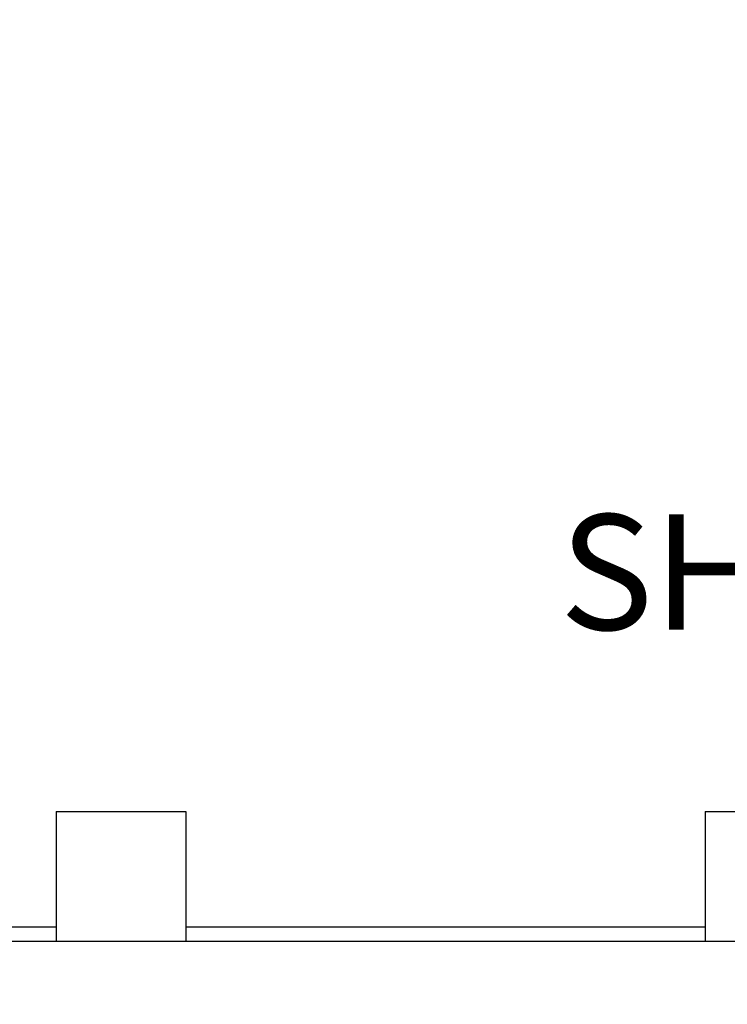
# Model space of a CAD drawing. Units: inches. Extents: x -48 to 50072, y 0 to 21068.
# Tile 4 of 75: x 163 to 212, y 210 to 278. Entities that reach past the tile are written whole.
import ezdxf

# ---------------------------------------------------------------- set-up
doc = ezdxf.new("R2010")
doc.units = ezdxf.units.IN
doc.header["$MEASUREMENT"] = 0
doc.layers.add('A-ANNO-DIMS', color=2, linetype='Continuous', lineweight=18)
doc.layers.add('C-PROP', color=7, linetype='Continuous', lineweight=25)
doc.styles.get("Standard").update_dxf_attribs({"font": 'arial.ttf'})
doc.dimstyles.get("Standard").update_dxf_attribs({"dimtxt": 8, "dimasz": 0.18, "dimexe": 0.18, "dimexo": 0.0625, "dimgap": 0.09, "dimtad": 0, "dimtih": 1, "dimtoh": 1, "dimdec": 1, "dimzin": 0, "dimdsep": 46, "dimlunit": 4, "dimtxsty": 'Standard', "dimblk": 'ARCHTICK', "dimcen": 0.09, "dimadec": 0, "dimazin": 0, "dimtfac": 1, "dimtdec": 1, "dimtofl": 0, "dimtmove": 0, "dimatfit": 3, "dimldrblk": 'ARCHTICK', "dimfxl": 1, "dimtolj": 1, "dimtzin": 0, "dimarcsym": 0})

# ---------------------------------------------------------------- blocks, each defined once
blk = doc.blocks.new('_ArchTick')
at = {"color": 0, "linetype": 'ByBlock', "const_width": 0.15}
blk.add_lwpolyline([(-0.5, -0.5), (0.5, 0.5)], dxfattribs=at)
blk = doc.blocks.new('*D52')
at = {"layer": 'A-ANNO-DIMS', "color": 0, "lineweight": -2, "transparency": 16777216}
for p, q in [((238.847, 252.654), (242.859, 252.654)), ((242.679, 252.654), (242.679, 243.897)), ((242.679, 226.686), (242.679, 235.444)), ((238.847, 226.686), (242.859, 226.686))]:
    blk.add_line(p, q, dxfattribs=at)
at = {"layer": 'Defpoints', "color": 0, "transparency": 16777216}
for p in [(238.784, 252.654), (242.679, 252.654), (238.784, 226.686)]:
    blk.add_point(p, dxfattribs=at)
at = {"layer": 'A-ANNO-DIMS', "color": 0, "lineweight": -2, "transparency": 16777216, "xscale": 0.18, "yscale": 0.18, "zscale": 0.18}
for p, rotation in [((242.679, 252.654), 90), ((242.679, 226.686), 270)]:
    blk.add_blockref('_ArchTick', p, dxfattribs=dict(at, rotation=rotation))
at = {"layer": 'A-ANNO-DIMS', "color": 0, "transparency": 16777216, "insert": (242.679, 239.67), "char_height": 8, "attachment_point": 5}
blk.add_mtext('\\A1;SHRUB A 26 TYP.', dxfattribs=at)
blk = doc.blocks.new('*D116')
at = {"layer": 'A-ANNO-DIMS', "color": 0, "lineweight": -2, "transparency": 16777216}
for p, q in [((18.017, 677.712), (18.017, 165.945)), ((216.017, 677.712), (216.017, 165.945)), ((18.017, 166.125), (108.458, 166.125)), ((216.017, 166.125), (125.576, 166.125))]:
    blk.add_line(p, q, dxfattribs=at)
at = {"layer": 'Defpoints', "color": 0, "transparency": 16777216}
for p in [(18.017, 677.775), (216.017, 677.775), (216.017, 166.125)]:
    blk.add_point(p, dxfattribs=at)
at = {"layer": 'A-ANNO-DIMS', "color": 0, "lineweight": -2, "transparency": 16777216, "xscale": 0.18, "yscale": 0.18, "zscale": 0.18, "rotation": 180}
blk.add_blockref('_ArchTick', (18.017, 166.125), dxfattribs=at)
at = {"layer": 'A-ANNO-DIMS', "color": 0, "lineweight": -2, "transparency": 16777216, "xscale": 0.18, "yscale": 0.18, "zscale": 0.18}
blk.add_blockref('_ArchTick', (216.017, 166.125), dxfattribs=at)
at = {"layer": 'A-ANNO-DIMS', "color": 0, "transparency": 16777216, "insert": (117.017, 166.125), "char_height": 8, "attachment_point": 5}
blk.add_mtext('\\A1;198', dxfattribs=at)

msp = doc.modelspace()

# ---------------------------------------------------------------- linework, layer by layer
at = {"layer": 'C-PROP'}
for p, q in [((165.389, 223.075), (165.389, 214.075)), ((165.389, 223.075), (174.389, 223.075)), ((174.389, 223.075), (174.389, 214.075)), ((210.389, 223.075), (210.389, 214.075)), ((210.389, 223.075), (544.517, 223.075)), ((39.243, 215.075), (165.389, 215.075)), ((174.389, 215.075), (210.389, 215.075)), ((39.243, 214.075), (165.389, 214.075)), ((165.389, 214.075), (174.389, 214.075)), ((174.389, 214.075), (210.389, 214.075)), ((210.389, 214.075), (553.517, 214.075))]:
    msp.add_line(p, q, dxfattribs=at)

# ---------------------------------------------------------------- dimensions: what is measured, and where the dimension line sits
at = {"layer": 'A-ANNO-DIMS'}
dim = msp.add_linear_dim(base=(216.017, 166.125), p1=(18.017, 677.775), p2=(216.017, 677.775), dimstyle='Standard', override={"dimdec": 0, "dimlfac": 1, "dimrnd": 0, "dimzin": 0, "dimdsep": 46, "dimlunit": 2}, dxfattribs=at)
dim.commit()
dim.dimension.update_dxf_attribs({"geometry": '*D116', "text_midpoint": (117.017, 166.125)})
dim = msp.add_linear_dim(base=(242.679, 252.654), p1=(238.784, 226.686), p2=(238.784, 252.654), angle=90, text='SHRUB A <> TYP.', dimstyle='Standard', override={"dimdec": 0, "dimlfac": 1, "dimrnd": 0, "dimzin": 0, "dimdsep": 46, "dimlunit": 2}, dxfattribs=at)
dim.commit()
dim.dimension.update_dxf_attribs({"geometry": '*D52', "text_midpoint": (242.679, 239.67)})

doc.saveas('drawing.dxf')
